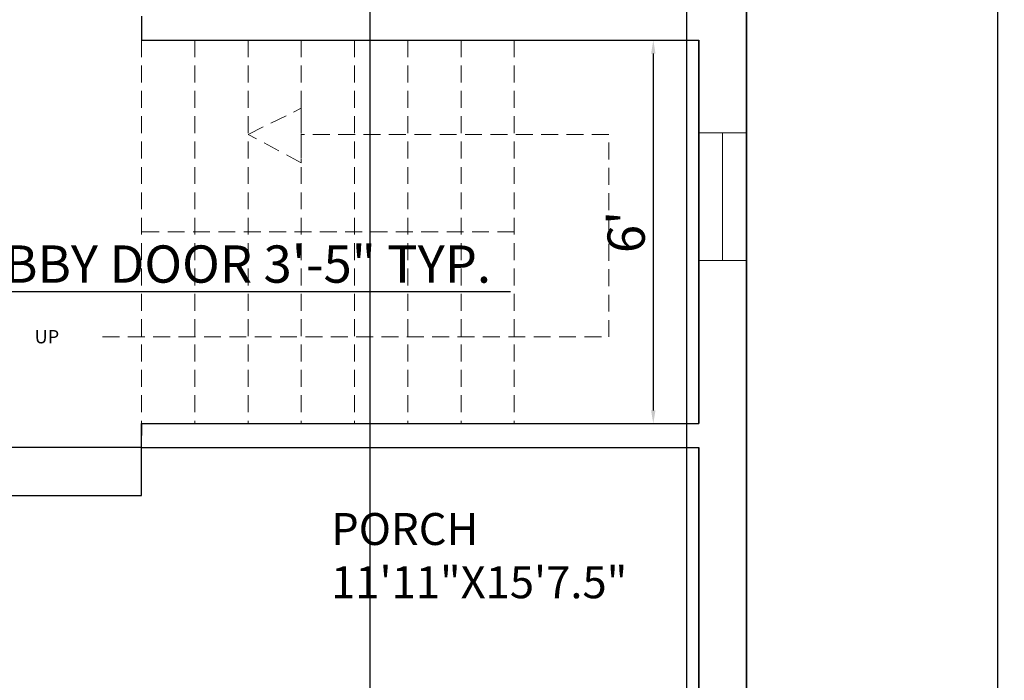
# Model space of a CAD drawing. Units: inches. Extents: x 1863 to 2938, y 1238 to 2492.
# Tile 6 of 12: x 2158 to 2343, y 1452 to 1576. Entities that reach past the tile are written whole.
import ezdxf

# ---------------------------------------------------------------- set-up
doc = ezdxf.new("R2010")
doc.units = ezdxf.units.IN
doc.linetypes.add('HIDDEN2', pattern=[4.7625, 3.175, -1.5875])
for name, color, linetype, lineweight in [('A-ANNO-DIMS', 2, 'Continuous', 18), ('A-ANNO-TEXT', 7, 'Continuous', 18), ('A-AREA-IDEN', 7, 'Continuous', 18), ('A-FLOR-STRS', 7, 'Continuous', 25), ('A-FLOR-STRS-HIDN', 253, 'HIDDEN2', 18), ('A-GLAZ', 4, 'Continuous', 18), ('A-WALL', 7, 'Continuous', 35)]:
    doc.layers.add(name, color=color, linetype=linetype, lineweight=lineweight)
doc.styles.get("Standard").update_dxf_attribs({"font": 'arial.ttf'})
doc.dimstyles.new('ISO-25', dxfattribs={"dimtxt": 7, "dimasz": 2.5, "dimexe": 1.25, "dimexo": 0.625, "dimtad": 1, "dimdec": 0, "dimlunit": 3, "dimtxsty": 'Standard', "dimcen": 2.5, "dimadec": 0, "dimazin": 0, "dimtfac": 1, "dimtdec": 0, "dimtmove": 0, "dimatfit": 3, "dimfxl": 1, "dimarcsym": 0})

# ---------------------------------------------------------------- blocks, each defined once
blk = doc.blocks.new('*D1')
at = {"layer": 'A-ANNO-DIMS', "color": 0, "lineweight": -2, "transparency": 16777216}
for p, q in [((2277.48, 1572.06), (2278.37, 1572.06)), ((2277.12, 1569.56), (2277.12, 1502.56)), ((2277.48, 1500.06), (2278.37, 1500.06))]:
    blk.add_line(p, q, dxfattribs=at)
at = {"layer": 'A-ANNO-DIMS', "color": 0, "transparency": 16777216}
for points in [[(2276.7, 1569.56), (2277.53, 1569.56), (2277.12, 1572.06)], [(2276.7, 1502.56), (2277.53, 1502.56), (2277.12, 1500.06)]]:
    blk.add_solid(points, dxfattribs=at)
at = {"layer": 'Defpoints', "color": 0, "transparency": 16777216}
for p in [(2276.86, 1572.06), (2276.86, 1500.06), (2277.12, 1500.06)]:
    blk.add_point(p, dxfattribs=at)
at = {"layer": 'A-ANNO-DIMS', "color": 0, "transparency": 16777216, "insert": (2272.92, 1536.06), "char_height": 7, "attachment_point": 5, "rotation": 90}
blk.add_mtext("6'", dxfattribs=at)
blk = doc.blocks.new('*D3')
at = {"layer": 'A-ANNO-DIMS', "color": 0, "lineweight": -2, "transparency": 16777216}
for p, q in [((2295.26, 2076.56), (2343.03, 2076.56)), ((2341.78, 2074.06), (2341.78, 1342.06)), ((2295.26, 1339.56), (2343.03, 1339.56))]:
    blk.add_line(p, q, dxfattribs=at)
at = {"layer": 'A-ANNO-DIMS', "color": 0, "transparency": 16777216}
for points in [[(2341.36, 2074.06), (2342.2, 2074.06), (2341.78, 2076.56)], [(2341.36, 1342.06), (2342.2, 1342.06), (2341.78, 1339.56)]]:
    blk.add_solid(points, dxfattribs=at)
at = {"layer": 'Defpoints', "color": 0, "transparency": 16777216}
for p in [(2294.64, 2076.56), (2294.64, 1339.56), (2341.78, 1339.56)]:
    blk.add_point(p, dxfattribs=at)
at = {"layer": 'A-ANNO-DIMS', "color": 0, "transparency": 16777216, "insert": (2337.58, 1708.06), "char_height": 7, "attachment_point": 5, "rotation": 90}
blk.add_mtext('61\'-5"', dxfattribs=at)
blk = doc.blocks.new('WIN-24')
for p, q in [((0, 24), (9, 24)), ((9, 24), (4.5, 24)), ((4.5, 24), (4.5, 0)), ((4.5, 0), (0, 0)), ((0, 0), (9, 0))]:
    blk.add_line(p, q)
blk = doc.blocks.new('STAIR-FLIGHT-HIDDEN')
for p, q in [((7.32, 72), (7.32, 0)), ((17.32, 72), (17.32, 0)), ((27.32, 72), (27.32, 0)), ((37.32, 72), (37.32, 0)), ((47.32, 72), (47.32, 0)), ((57.32, 72), (57.32, 0)), ((67.32, 72), (67.32, 0)), ((77.32, 72), (77.32, 0)), ((27.32, 54.32), (37.32, 59.21)), ((37.32, 59.21), (37.32, 59.21)), ((37.32, 59.21), (37.32, 48.95)), ((37.32, 48.95), (27.32, 54.32)), ((95.06, 54.32), (37.32, 54.32)), ((95.06, 16.28), (95.06, 54.32)), ((77.32, 36), (7.32, 36)), ((0, 16.28), (95.06, 16.28))]:
    blk.add_line(p, q)
blk = doc.blocks.new('*D56')
at = {"layer": 'A-ANNO-DIMS', "color": 0, "lineweight": -2, "transparency": 16777216}
for p, q in [((2095.74, 1530.4), (2095.74, 1523.62)), ((2136.81, 1530.4), (2136.81, 1523.62)), ((2098.24, 1524.87), (2134.31, 1524.87)), ((2136.81, 1524.87), (2250.3, 1524.87))]:
    blk.add_line(p, q, dxfattribs=at)
at = {"layer": 'A-ANNO-DIMS', "color": 0, "transparency": 16777216}
for points in [[(2098.24, 1525.28), (2098.24, 1524.45), (2095.74, 1524.87)], [(2134.31, 1525.28), (2134.31, 1524.45), (2136.81, 1524.87)]]:
    blk.add_solid(points, dxfattribs=at)
at = {"layer": 'Defpoints', "color": 0, "transparency": 16777216}
for p in [(2095.74, 1531.03), (2136.81, 1531.03), (2136.81, 1524.87)]:
    blk.add_point(p, dxfattribs=at)
at = {"layer": 'A-ANNO-DIMS', "color": 0, "transparency": 16777216, "insert": (2194.8, 1529.12), "char_height": 7, "attachment_point": 5}
blk.add_mtext('LOBBY DOOR 3\'-5" TYP.', dxfattribs=at)
blk = doc.blocks.new('*D58')
at = {"layer": 'A-ANNO-DIMS', "color": 0, "lineweight": -2, "transparency": 16777216}
for p, q in [((2223.92, 1623.6), (2223.92, 1243.07)), ((2283.38, 1624.45), (2283.38, 1243.07)), ((2226.42, 1244.32), (2280.88, 1244.32))]:
    blk.add_line(p, q, dxfattribs=at)
at = {"layer": 'A-ANNO-DIMS', "color": 0, "transparency": 16777216}
for points in [[(2226.42, 1244.74), (2226.42, 1243.91), (2223.92, 1244.32)], [(2280.88, 1244.74), (2280.88, 1243.91), (2283.38, 1244.32)]]:
    blk.add_solid(points, dxfattribs=at)
at = {"layer": 'Defpoints', "color": 0, "transparency": 16777216}
for p in [(2223.92, 1624.22), (2283.38, 1625.07), (2283.38, 1244.32)]:
    blk.add_point(p, dxfattribs=at)
at = {"layer": 'A-ANNO-DIMS', "color": 0, "transparency": 16777216, "insert": (2253.65, 1248.57), "char_height": 7, "attachment_point": 5}
blk.add_mtext('4\'-11 1/2"', dxfattribs=at)

msp = doc.modelspace()

# ---------------------------------------------------------------- linework, layer by layer
at = {"layer": 'A-FLOR-STRS'}
for p, q in [((2181.02, 1576.56), (2181.02, 1572.06)), ((2181.02, 1572.06), (2285.64, 1572.06)), ((2181.02, 1500.06), (2285.64, 1500.06)), ((2181.02, 1495.56), (2181.02, 1500.06)), ((2181.02, 1500.06), (2181.02, 1497.81)), ((2181.02, 1495.56), (2149.14, 1495.56)), ((2181.02, 1495.56), (2285.64, 1495.56)), ((2181.02, 1495.56), (2181.02, 1495.56)), ((2181.02, 1486.56), (2181.02, 1495.56)), ((2149.14, 1486.56), (2181.02, 1486.56))]:
    msp.add_line(p, q, dxfattribs=at)
at = {"layer": 'A-WALL'}
for p, q in [((2294.64, 2076.56), (2294.64, 1495.56)), ((2285.64, 1572.06), (2285.64, 1500.06)), ((2285.64, 1339.56), (2285.64, 1495.56)), ((2294.64, 1495.56), (2294.64, 1339.56))]:
    msp.add_line(p, q, dxfattribs=at)

# ---------------------------------------------------------------- block references
at = {"layer": 'A-FLOR-STRS-HIDN'}
msp.add_blockref('STAIR-FLIGHT-HIDDEN', (2173.7, 1500.06), dxfattribs=at)
at = {"layer": 'A-GLAZ', "rotation": 180}
msp.add_blockref('WIN-24', (2294.64, 1554.67), dxfattribs=at)

# ---------------------------------------------------------------- texts
at = {"layer": 'A-ANNO-TEXT', "insert": (2160.94, 1517.64), "char_height": 2.5, "attachment_point": 1}
msp.add_mtext_dynamic_manual_height_columns('UP', width=10.4918, gutter_width=12.5, heights=[0], dxfattribs=at)
at = {"layer": 'A-AREA-IDEN', "insert": (2216.62, 1483.28), "char_height": 6, "attachment_point": 1}
msp.add_mtext_dynamic_manual_height_columns('PORCH\\P11\'11"X15\'7.5"', width=92.3154, gutter_width=12.5, heights=[0], dxfattribs=at)

# ---------------------------------------------------------------- dimensions: what is measured, and where the dimension line sits
at = {"layer": 'A-ANNO-DIMS'}
for base, p1, p2, picture, middle in [((2341.78, 1339.56), (2294.64, 2076.56), (2294.64, 1339.56), '*D3', (2337.58, 1708.06)), ((2277.12, 1500.06), (2276.86, 1572.06), (2276.86, 1500.06), '*D1', (2272.92, 1536.06))]:
    dim = msp.add_linear_dim(base=base, p1=p1, p2=p2, angle=90, dimstyle='ISO-25', override={"dimclrd": 0, "dimclre": 0, "dimclrt": 0}, dxfattribs=at)
    dim.commit()
    dim.dimension.update_dxf_attribs({"geometry": picture, "text_midpoint": middle})
dim = msp.add_linear_dim(base=(2283.38, 1244.32), p1=(2223.92, 1624.22), p2=(2283.38, 1625.07), dimstyle='ISO-25', override={"dimdec": 1, "dimlfac": 1, "dimrnd": 0, "dimzin": 1, "dimdsep": 46, "dimlunit": 4, "dimfrac": 2}, dxfattribs=at)
dim.commit()
dim.dimension.update_dxf_attribs({"geometry": '*D58', "text_midpoint": (2253.65, 1248.57)})
dim = msp.add_linear_dim(base=(2136.81, 1524.87), p1=(2095.74, 1531.03), p2=(2136.81, 1531.03), text='LOBBY DOOR <> TYP.', dimstyle='ISO-25', override={"dimdec": 1, "dimlfac": 1, "dimrnd": 0, "dimzin": 1, "dimdsep": 46, "dimlunit": 4, "dimfrac": 2}, dxfattribs=at)
dim.commit()
dim.dimension.update_dxf_attribs({"geometry": '*D56', "text_midpoint": (2194.8, 1529.12)})

doc.saveas('drawing.dxf')
